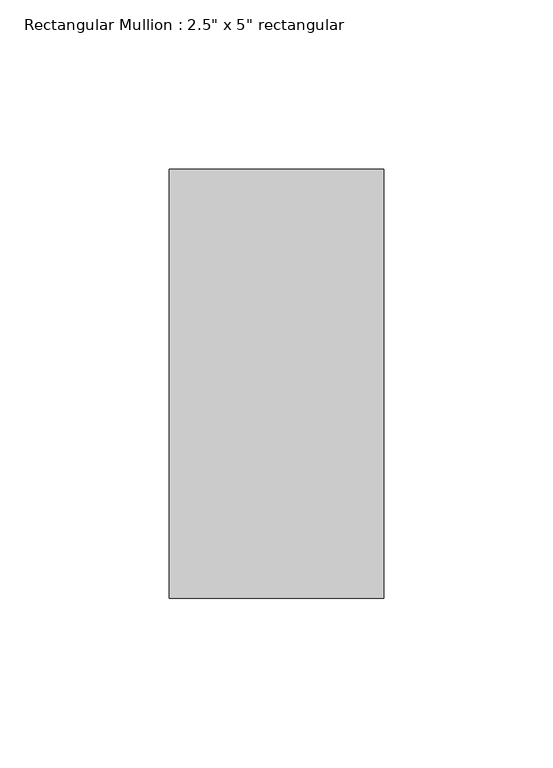
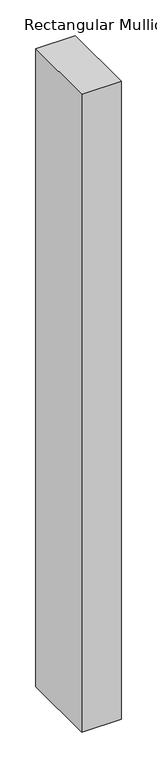
"""IFC4 building model written with IfcOpenShell, lengths in millimetres: member geometry."""

from ifc_helpers import new_model, si_unit, frame, origin, place, context, project, spatial, polyline, outline, extrude, source, transform, mapped, element, save


def member_96c24052(model_context):
    return source(origin(), model_context, "Body", "SweptSolid", [
        extrude(outline(polyline([(0.0, 63.5), (0.0, -63.5), (-63.5, -63.5), (-63.5, 63.5), (0.0, 63.5)])), frame((0.0, 0.0, -1084.1873156), z_axis=(0.0, 0.0, 1.0), x_axis=(1.0, 0.0, 0.0)), (0.0, 0.0, 1.0), 1084.1873156),
    ])


if __name__ == "__main__":
    model = new_model("IFC4")
    model_context = context("Model", 3, world=origin())
    ifc_project = project(units=[si_unit("LENGTHUNIT", "METRE", prefix="MILLI")], contexts=[model_context])
    site = spatial("IfcSite", under=ifc_project)
    building = spatial("IfcBuilding", under=site)
    placement = place(None, origin())
    member_shape = member_96c24052(model_context)
    element("IfcMember", 1, ObjectType="Rectangular Mullion : 2.5\" x 5\" rectangular", at=placement, inside=building, context=model_context, shape_type="MappedRepresentation", body=[
        mapped(member_shape, transform((0.0, 0.0, 0.0), x_axis=(1.0, 0.0, 0.0), y_axis=(0.0, 1.0, 0.0), z_axis=(0.0, 0.0, 1.0))),
    ])
    save(model, "model.ifc")

# Revit data of these elements
# Type "Rectangular Mullion : 2.5\" x 5\" rectangular"
#   built-in parameter 1007304 = 0.416667 (stored number, unit not read)
#   built-in parameter 1007301 = 0.104167 (stored number, unit not read)
#   built-in parameter 1007300 = 0.104167 (stored number, unit not read)
# Element 1 (IfcMember, "Rectangular Mullion : 2.5\" x 5\" rectangular")
#   Materials on its faces: "Aluminum"
# Materials
#   "Aluminum": class "Metal", colour RGB 247 247 247, transparency 0, Description = "Aluminum 6061", Cost = 0
